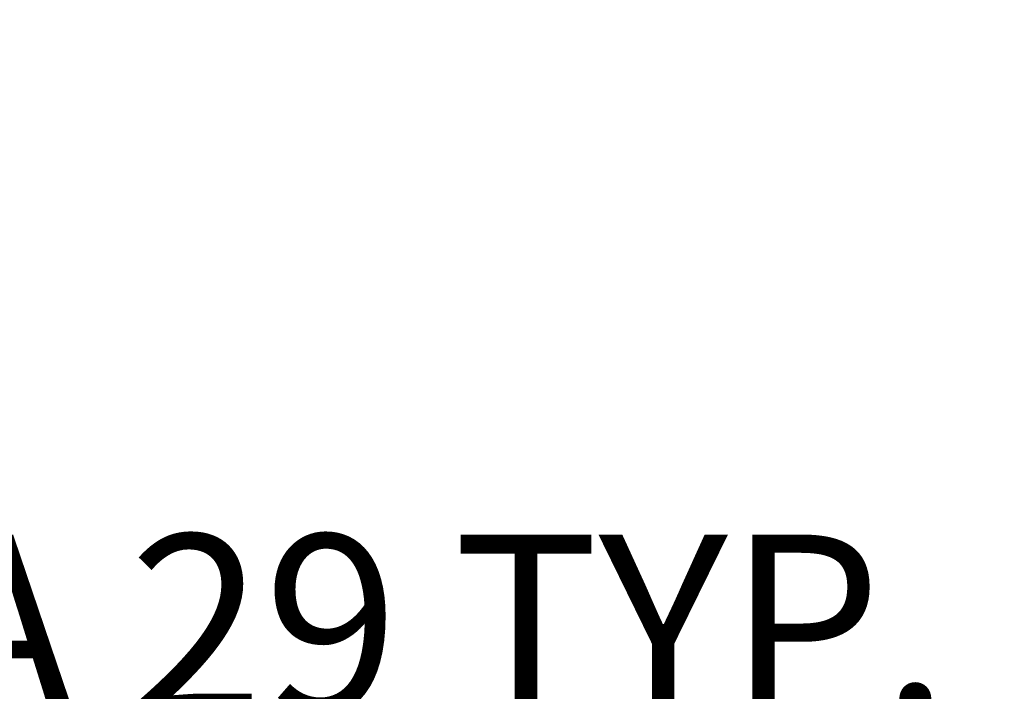
# Model space of a CAD drawing. Units: inches. Extents: x 1704 to 6393, y -157 to 1172.
# Tile 101 of 122: x 2561 to 2594, y 1034 to 1056. Entities that reach past the tile are written whole.
import ezdxf

# ---------------------------------------------------------------- set-up
doc = ezdxf.new("R2010")
doc.units = ezdxf.units.IN
doc.header["$MEASUREMENT"] = 0
doc.layers.add('A-ANNO-DIMS', color=7, linetype='Continuous', lineweight=13)
doc.styles.get("Standard").update_dxf_attribs({"font": 'arial.ttf'})
doc.dimstyles.get("Standard").update_dxf_attribs({"dimtxt": 6, "dimasz": 2, "dimexe": 0.18, "dimexo": 0.0625, "dimgap": 0.09, "dimtad": 0, "dimtih": 1, "dimtoh": 1, "dimdec": 1, "dimzin": 0, "dimdsep": 46, "dimlunit": 3, "dimtxsty": 'Standard', "dimblk": 'ARCHTICK', "dimcen": 0.09, "dimadec": 0, "dimazin": 0, "dimtfac": 1, "dimtdec": 1, "dimtofl": 0, "dimtmove": 0, "dimatfit": 3, "dimfxl": 1, "dimtolj": 1, "dimtzin": 0, "dimarcsym": 0})

# ---------------------------------------------------------------- blocks, each defined once
blk = doc.blocks.new('_ArchTick')
at = {"color": 0, "linetype": 'ByBlock', "const_width": 0.15}
blk.add_lwpolyline([(-0.5, -0.5), (0.5, 0.5)], dxfattribs=at)
blk = doc.blocks.new('*D88')
at = {"layer": 'A-ANNO-DIMS', "color": 0, "lineweight": -2, "transparency": 16777216}
for p, q in [((2596.639, 1031.77), (2596.639, 1036.222)), ((2625.54, 1031.77), (2625.54, 1036.222)), ((2596.639, 1036.042), (2594.639, 1036.042)), ((2625.54, 1036.042), (2596.639, 1036.042))]:
    blk.add_line(p, q, dxfattribs=at)
at = {"layer": 'Defpoints', "color": 0, "lineweight": -3, "transparency": 16777216}
for p in [(2596.639, 1036.042), (2596.639, 1031.707), (2625.54, 1031.707)]:
    blk.add_point(p, dxfattribs=at)
at = {"layer": 'A-ANNO-DIMS', "color": 0, "lineweight": -2, "transparency": 16777216, "xscale": 2, "yscale": 2, "zscale": 2, "rotation": 180}
blk.add_blockref('_ArchTick', (2596.639, 1036.042), dxfattribs=at)
at = {"layer": 'A-ANNO-DIMS', "color": 0, "lineweight": -2, "transparency": 16777216, "xscale": 2, "yscale": 2, "zscale": 2}
blk.add_blockref('_ArchTick', (2625.54, 1036.042), dxfattribs=at)
at = {"layer": 'A-ANNO-DIMS', "color": 0, "transparency": 16777216, "insert": (2560.165, 1036.042), "char_height": 6, "attachment_point": 5}
blk.add_mtext('\\A1;SHRUB A 29 TYP.', dxfattribs=at)
blk = doc.blocks.new('*D92')
at = {"layer": 'A-ANNO-DIMS', "color": 0, "lineweight": -2, "transparency": 16777216}
for p, q in [((2073.349, 895.275), (2073.349, 1105.287)), ((2605.349, 895.275), (2605.349, 1105.287)), ((2073.349, 1105.107), (2332.661, 1105.107)), ((2605.349, 1105.107), (2346.036, 1105.107))]:
    blk.add_line(p, q, dxfattribs=at)
at = {"layer": 'Defpoints', "color": 0, "lineweight": -3, "transparency": 16777216}
for p in [(2605.349, 1105.107), (2073.349, 895.213), (2605.349, 895.213)]:
    blk.add_point(p, dxfattribs=at)
at = {"layer": 'A-ANNO-DIMS', "color": 0, "lineweight": -2, "transparency": 16777216, "xscale": 2, "yscale": 2, "zscale": 2, "rotation": 180}
blk.add_blockref('_ArchTick', (2073.349, 1105.107), dxfattribs=at)
at = {"layer": 'A-ANNO-DIMS', "color": 0, "lineweight": -2, "transparency": 16777216, "xscale": 2, "yscale": 2, "zscale": 2}
blk.add_blockref('_ArchTick', (2605.349, 1105.107), dxfattribs=at)
at = {"layer": 'A-ANNO-DIMS', "color": 0, "transparency": 16777216, "insert": (2339.349, 1105.107), "char_height": 6, "attachment_point": 5}
blk.add_mtext('\\A1;532', dxfattribs=at)
blk = doc.blocks.new('*D103')
at = {"layer": 'A-ANNO-DIMS', "color": 0, "lineweight": -2, "transparency": 16777216}
for p, q in [((2551.349, 711.275), (2551.349, 1105.287)), ((2597.349, 711.275), (2597.349, 1105.287)), ((2551.349, 1105.107), (2569.842, 1105.107)), ((2597.349, 1105.107), (2578.855, 1105.107))]:
    blk.add_line(p, q, dxfattribs=at)
at = {"layer": 'Defpoints', "color": 0, "lineweight": -3, "transparency": 16777216}
for p in [(2597.349, 1105.107), (2551.349, 711.213), (2597.349, 711.213)]:
    blk.add_point(p, dxfattribs=at)
at = {"layer": 'A-ANNO-DIMS', "color": 0, "lineweight": -2, "transparency": 16777216, "xscale": 2, "yscale": 2, "zscale": 2, "rotation": 180}
blk.add_blockref('_ArchTick', (2551.349, 1105.107), dxfattribs=at)
at = {"layer": 'A-ANNO-DIMS', "color": 0, "lineweight": -2, "transparency": 16777216, "xscale": 2, "yscale": 2, "zscale": 2}
blk.add_blockref('_ArchTick', (2597.349, 1105.107), dxfattribs=at)
at = {"layer": 'A-ANNO-DIMS', "color": 0, "transparency": 16777216, "insert": (2574.349, 1105.107), "char_height": 6, "attachment_point": 5}
blk.add_mtext('\\A1;46', dxfattribs=at)

msp = doc.modelspace()

# ---------------------------------------------------------------- dimensions: what is measured, and where the dimension line sits
at = {"layer": 'A-ANNO-DIMS'}
for base, p1, p2, picture, middle in [((2605.349, 1105.107), (2073.349, 895.213), (2605.349, 895.213), '*D92', (2339.349, 1105.107)), ((2597.349, 1105.107), (2551.349, 711.213), (2597.349, 711.213), '*D103', (2574.349, 1105.107))]:
    dim = msp.add_linear_dim(base=base, p1=p1, p2=p2, dimstyle='Standard', override={"dimdec": 0, "dimlfac": 1, "dimrnd": 0, "dimzin": 0, "dimdsep": 46, "dimlunit": 2}, dxfattribs=at)
    dim.commit()
    dim.dimension.update_dxf_attribs({"geometry": picture, "text_midpoint": middle})
dim = msp.add_linear_dim(base=(2596.639, 1036.042), p1=(2625.54, 1031.707), p2=(2596.639, 1031.707), angle=180, text='SHRUB A <> TYP.', dimstyle='Standard', override={"dimdec": 0, "dimlfac": 1, "dimrnd": 0, "dimzin": 0, "dimdsep": 46, "dimlunit": 2}, dxfattribs=at)
dim.commit()
dim.dimension.update_dxf_attribs({"geometry": '*D88', "text_midpoint": (2560.165, 1036.042)})

doc.saveas('drawing.dxf')
